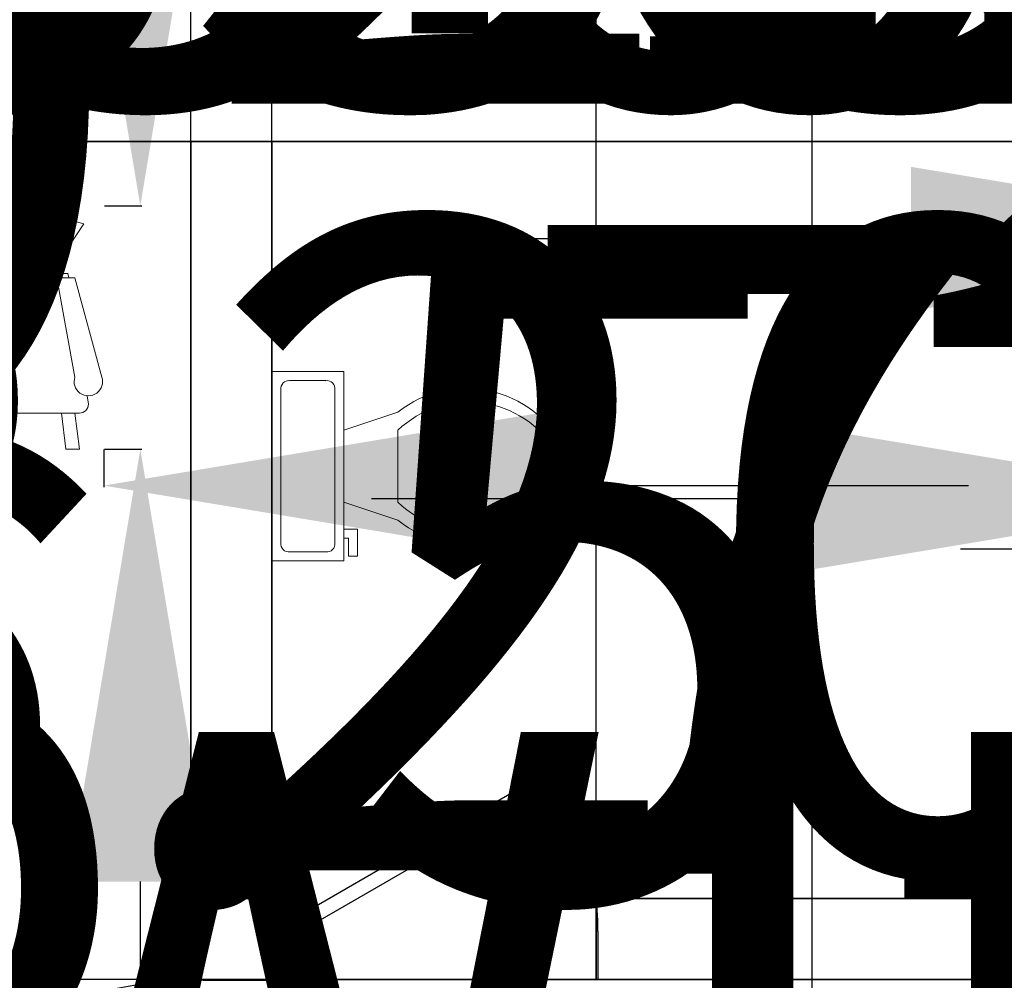
# Model space of a CAD drawing. Units: inches. Extents: x -307 to 2141, y -58 to 895.
# Tile 20 of 28: x 666 to 776, y 589 to 696. Entities that reach past the tile are written whole.
import ezdxf

# ---------------------------------------------------------------- set-up
doc = ezdxf.new("R2010")
doc.units = ezdxf.units.IN
doc.header["$MEASUREMENT"] = 0
for name, color, linetype, lineweight in [('A-ANNO-DIMS', 2, 'Continuous', 18), ('A-DOOR', 3, 'Continuous', 25), ('A-FLOR-FIXT', 9, 'Continuous', 18), ('A-FURN', 8, 'Continuous', 18), ('A-WALL', 7, 'Continuous', 35)]:
    doc.layers.add(name, color=color, linetype=linetype, lineweight=lineweight)
doc.styles.get("Standard").update_dxf_attribs({"font": 'arial.ttf'})
doc.dimstyles.get("Standard").update_dxf_attribs({"dimtxt": 72, "dimasz": 48, "dimexe": 0.18, "dimexo": 0.0625, "dimgap": 0.09, "dimtad": 0, "dimtih": 1, "dimtoh": 1, "dimdec": 0, "dimrnd": 48, "dimzin": 0, "dimdsep": 46, "dimlunit": 3, "dimtxsty": 'Standard', "dimcen": 0.09, "dimadec": 0, "dimazin": 0, "dimtfac": 1, "dimtdec": 0, "dimtofl": 0, "dimtmove": 0, "dimatfit": 3, "dimfxl": 1, "dimtolj": 1, "dimtzin": 0, "dimarcsym": 0})

# ---------------------------------------------------------------- blocks, each defined once
blk = doc.blocks.new('*U3')
for p, q in [((-40, 0), (-40, 6)), ((0, 0), (0, 6))]:
    blk.add_line(p, q)
blk.add_lwpolyline([(0, 0), (-34.641, -20), (-35.516, -18.484), (-0.875, 1.516)], close=True)
blk.add_arc((0, 0), 40, 180, 210)
blk = doc.blocks.new('*U4')
for p, q in [((-40, 0), (-40, 6)), ((0, 0), (0, 6))]:
    blk.add_line(p, q)
blk.add_lwpolyline([(0, 0), (-34.64, -20), (-35.52, -18.48), (-0.88, 1.52)], close=True)
blk.add_arc((0, 0), 40, 180, 210)
blk = doc.blocks.new('Toilet - top')
for p, q in [((9.5, -6), (9.5, -2)), ((-10, -8.5), (-8, -8.5)), ((-10, -9.5), (-10, -8.5)), ((-8, -8.5), (-8, -8)), ((-7, -8), (-7, -9.5)), ((-4, -8), (-6, -14)), ((4, -8), (6, -14)), ((-7, -9.5), (-10, -9.5)), ((4, -14), (-4, -14))]:
    blk.add_line(p, q)
blk.add_lwpolyline([(10.5, -8), (10.5, 0), (-10.5, 0), (-10.5, -8)], close=True)
for points in [[(8.5, -1), (-8.5, -1)], [(-9.5, -2), (-9.5, -6)], [(-8.5, -7), (8.5, -7)]]:
    blk.add_lwpolyline(points)
for centre, radius, start, end in [((-8.62, -1.88), 0.884, 81.8699, 188.1301), ((8.62, -1.88), 0.884, 351.8699, 98.1301), ((-8.62, -6.12), 0.884, 171.8699, 278.1301), ((8.62, -6.12), 0.884, 261.8699, 8.1301), ((3.52, -21.58), 12.17, 141.4691, 247.9714), ((4.2, -21.82), 11.33, 136.3677, 238.9468), ((-3.52, -21.58), 12.17, 292.0284, 38.5307), ((-4.2, -21.82), 11.33, 301.053, 43.6321), ((0, -27.88), 4, 245.7318, 294.2682), ((0, -29), 4, 254.8605, 285.1395)]:
    blk.add_arc(centre, radius, start, end)
blk = doc.blocks.new('Chair - Rocking')
for p, q in [((-8, -4.5), (-10, -1.5)), ((8, -4.5), (10, -1.5)), ((-4.5, -7), (-4.96674, -4.19951)), ((-4, -7), (-4.40532, -4.16272)), ((-1.5, -4.05012), (-1.5, -7)), ((-1, -7), (-1, -4.05012)), ((1, -7), (1, -4.04655)), ((1.5, -4.05012), (1.5, -7)), ((4, -7), (4.40187, -4.18694)), ((4.5, -7), (4.96761, -4.19437)), ((-7.5, -4.5), (-7, -7)), ((-6.5, -7), (-7.02225, -4.43)), ((6.5, -7), (7, -4.4057)), ((7.5, -4.5), (7, -7)), ((-9, -7.5), (-12, -18.49999)), ((-7, -7.5), (-9, -7.5)), ((-9, -18.49999), (-7, -7.5)), ((-8.23428, -6.99939), (-8.3093, -7.47958)), ((-8.23041, -7), (8.23915, -7)), ((7, -7.5), (9, -7.5)), ((9, -18.49999), (7, -7.5)), ((8.31071, -7.48854), (8.23449, -7.00073)), ((9, -7.5), (12, -18.49999)), ((-10.36644, -20.64523), (-10.5, -21.49999)), ((10.5, -21.49999), (10.3575, -20.58798)), ((-9, -22.49999), (-9.5, -26.49999)), ((0, -22.49999), (-9.5, -22.49999)), ((-8, -26.49999), (-7.5, -22.49999)), ((0, -22.49999), (9.5, -22.49999)), ((8, -26.49999), (7.5, -22.49999)), ((9, -22.49999), (9.5, -26.49999)), ((-9.5, -26.49999), (-8, -26.49999)), ((9.5, -26.49999), (8, -26.49999))]:
    blk.add_line(p, q)
for centre, radius, start, end in [((0, -34.08333), 34.08333, 72.93847, 107.0615), ((0, -68.25004), 64.25, 93.92211, 97.15267), ((0, -68.25004), 64.25, 82.84733, 93.92211), ((-10.5, -18.99999), 1.58114, 161.5651, 18.43495), ((10.5, -18.99999), 1.58114, 161.5651, 18.43495), ((-9.5, -21.49999), 1, 180, 270), ((9.5, -21.49999), 1, 270, 0)]:
    blk.add_arc(centre, radius, start, end)
blk = doc.blocks.new('*D26')
at = {"layer": 'A-ANNO-DIMS', "color": 0, "lineweight": -2, "transparency": 16777216}
for p, q in [((565.34, 584.2), (565.34, 572.08)), ((645.34, 584.2), (645.34, 572.08)), ((517.34, 572.26), (469.34, 572.26)), ((693.34, 572.26), (741.34, 572.26))]:
    blk.add_line(p, q, dxfattribs=at)
at = {"layer": 'A-ANNO-DIMS', "color": 0, "transparency": 16777216}
for points in [[(517.34, 580.26), (517.34, 564.26), (565.34, 572.26)], [(693.34, 580.26), (693.34, 564.26), (645.34, 572.26)]]:
    blk.add_solid(points, dxfattribs=at)
at = {"layer": 'Defpoints', "color": 0, "transparency": 16777216}
for p in [(565.34, 584.26), (645.34, 584.26), (565.34, 572.26)]:
    blk.add_point(p, dxfattribs=at)
at = {"layer": 'A-ANNO-DIMS', "color": 0, "transparency": 16777216, "insert": (178.23, 572.26), "char_height": 72, "attachment_point": 5}
blk.add_mtext('\\A1;BED 80 TYP.', dxfattribs=at)
blk = doc.blocks.new('*D30')
at = {"layer": 'A-ANNO-DIMS', "color": 0, "lineweight": -2, "transparency": 16777216}
for p, q in [((570.74, 532.83), (570.74, 580.83)), ((570.74, 580.83), (618.74, 580.83)), ((565.4, 484.83), (570.92, 484.83)), ((565.4, 448.83), (570.92, 448.83)), ((570.74, 400.83), (570.74, 352.83))]:
    blk.add_line(p, q, dxfattribs=at)
at = {"layer": 'A-ANNO-DIMS', "color": 0, "transparency": 16777216}
for points in [[(562.74, 532.83), (578.74, 532.83), (570.74, 484.83)], [(562.74, 400.83), (578.74, 400.83), (570.74, 448.83)]]:
    blk.add_solid(points, dxfattribs=at)
at = {"layer": 'Defpoints', "color": 0, "transparency": 16777216}
for p in [(565.34, 484.83), (570.74, 484.83), (565.34, 448.83)]:
    blk.add_point(p, dxfattribs=at)
at = {"layer": 'A-ANNO-DIMS', "color": 0, "transparency": 16777216, "insert": (1030.17, 580.83), "char_height": 72, "attachment_point": 5}
blk.add_mtext('\\A1;WINDOW 36 TYP.', dxfattribs=at)
blk = doc.blocks.new('*D32')
at = {"layer": 'A-ANNO-DIMS', "color": 0, "lineweight": -2, "transparency": 16777216}
for p, q in [((813.29, 682.28), (813.29, 671.36)), ((885.29, 682.28), (885.29, 671.36)), ((765.29, 671.54), (717.29, 671.54)), ((933.29, 671.54), (981.29, 671.54))]:
    blk.add_line(p, q, dxfattribs=at)
at = {"layer": 'A-ANNO-DIMS', "color": 0, "transparency": 16777216}
for points in [[(765.29, 679.54), (765.29, 663.54), (813.29, 671.54)], [(933.29, 679.54), (933.29, 663.54), (885.29, 671.54)]]:
    blk.add_solid(points, dxfattribs=at)
at = {"layer": 'Defpoints', "color": 0, "transparency": 16777216}
for p in [(813.29, 682.34), (885.29, 682.34), (885.29, 671.54)]:
    blk.add_point(p, dxfattribs=at)
at = {"layer": 'A-ANNO-DIMS', "color": 0, "transparency": 16777216, "insert": (1392.73, 671.54), "char_height": 72, "attachment_point": 5}
blk.add_mtext('\\A1;WINDOW 72 TYP.', dxfattribs=at)
blk = doc.blocks.new('*D36')
at = {"layer": 'A-ANNO-DIMS', "color": 0, "lineweight": -2, "transparency": 16777216}
for p, q in [((871.71, 562.4), (871.76, 610.4)), ((876.55, 514.4), (871.47, 514.4)), ((876.51, 481.35), (871.44, 481.36)), ((871.56, 433.36), (871.51, 385.36)), ((871.51, 385.36), (823.51, 385.36))]:
    blk.add_line(p, q, dxfattribs=at)
at = {"layer": 'A-ANNO-DIMS', "color": 0, "transparency": 16777216}
for points in [[(863.71, 562.41), (879.71, 562.4), (871.65, 514.4)], [(863.56, 433.37), (879.56, 433.35), (871.62, 481.36)]]:
    blk.add_solid(points, dxfattribs=at)
at = {"layer": 'Defpoints', "color": 0, "transparency": 16777216}
for p in [(876.61, 514.4), (871.62, 481.36), (876.57, 481.35)]:
    blk.add_point(p, dxfattribs=at)
at = {"layer": 'A-ANNO-DIMS', "color": 0, "transparency": 16777216, "insert": (548.95, 385.36), "char_height": 72, "attachment_point": 5}
blk.add_mtext('\\A1;WC 33 TYP.', dxfattribs=at)
blk = doc.blocks.new('*D37')
at = {"layer": 'A-ANNO-DIMS', "color": 0, "lineweight": -2, "transparency": 16777216}
for p, q in [((828.62, 519.41), (780.62, 519.46)), ((876.61, 514.46), (876.62, 519.54)), ((897.61, 514.44), (897.62, 519.51)), ((945.62, 519.28), (993.62, 519.22))]:
    blk.add_line(p, q, dxfattribs=at)
at = {"layer": 'A-ANNO-DIMS', "color": 0, "transparency": 16777216}
for points in [[(828.63, 527.41), (828.61, 511.41), (876.62, 519.36)], [(945.63, 527.28), (945.61, 511.28), (897.62, 519.33)]]:
    blk.add_solid(points, dxfattribs=at)
at = {"layer": 'Defpoints', "color": 0, "transparency": 16777216}
for p in [(876.62, 519.36), (876.61, 514.4), (897.61, 514.38)]:
    blk.add_point(p, dxfattribs=at)
at = {"layer": 'A-ANNO-DIMS', "color": 0, "transparency": 16777216, "insert": (604.68, 519.46), "char_height": 72, "attachment_point": 5}
blk.add_mtext('\\A1;21 TYP.', dxfattribs=at)
blk = doc.blocks.new('*D42')
at = {"layer": 'A-ANNO-DIMS', "color": 0, "lineweight": -2, "transparency": 16777216}
for p, q in [((880.26, 543.86), (928.25, 544.87)), ((822.3, 541.2), (822.27, 542.82)), ((832.3, 541.41), (832.27, 543.03)), ((774.28, 541.63), (726.29, 540.62))]:
    blk.add_line(p, q, dxfattribs=at)
at = {"layer": 'A-ANNO-DIMS', "color": 0, "transparency": 16777216}
for points in [[(880.09, 551.86), (880.43, 535.86), (832.27, 542.85)], [(774.11, 549.63), (774.45, 533.63), (822.27, 542.64)]]:
    blk.add_solid(points, dxfattribs=at)
at = {"layer": 'Defpoints', "color": 0, "transparency": 16777216}
for p in [(832.27, 542.85), (832.3, 541.35), (822.3, 541.14)]:
    blk.add_point(p, dxfattribs=at)
at = {"layer": 'A-ANNO-DIMS', "color": 0, "transparency": 16777216, "insert": (1192.89, 544.87), "char_height": 72, "attachment_point": 5}
blk.add_mtext('\\A1;FAUCET 10', dxfattribs=at)
blk = doc.blocks.new('*D43')
at = {"layer": 'A-ANNO-DIMS', "color": 0, "lineweight": -2, "transparency": 16777216}
for p, q in [((818.79, 637.09), (770.79, 637.09)), ((819.79, 589.1), (818.79, 637.09)), ((822.24, 541.14), (820.62, 541.1)), ((822.38, 534.64), (820.76, 534.61)), ((821.95, 486.62), (822.96, 438.63))]:
    blk.add_line(p, q, dxfattribs=at)
at = {"layer": 'A-ANNO-DIMS', "color": 0, "transparency": 16777216}
for points in [[(827.79, 589.27), (811.8, 588.93), (820.8, 541.11)], [(829.95, 486.79), (813.95, 486.45), (820.94, 534.61)]]:
    blk.add_solid(points, dxfattribs=at)
at = {"layer": 'Defpoints', "color": 0, "transparency": 16777216}
for p in [(820.8, 541.11), (822.3, 541.14), (822.44, 534.64)]:
    blk.add_point(p, dxfattribs=at)
at = {"layer": 'A-ANNO-DIMS', "color": 0, "transparency": 16777216, "insert": (747.39, 637.09), "char_height": 72, "attachment_point": 5}
blk.add_mtext('\\A1;7', dxfattribs=at)
blk = doc.blocks.new('*D44')
at = {"layer": 'A-ANNO-DIMS', "color": 0, "lineweight": -2, "transparency": 16777216}
for p, q in [((815.33, 520.71), (815.41, 516.91)), ((839.87, 521.22), (839.95, 517.42)), ((887.94, 518.61), (935.93, 519.62)), ((767.41, 516.08), (719.42, 515.07))]:
    blk.add_line(p, q, dxfattribs=at)
at = {"layer": 'A-ANNO-DIMS', "color": 0, "transparency": 16777216}
for points in [[(887.77, 526.61), (888.11, 510.61), (839.95, 517.6)], [(767.25, 524.08), (767.58, 508.08), (815.4, 517.09)]]:
    blk.add_solid(points, dxfattribs=at)
at = {"layer": 'Defpoints', "color": 0, "transparency": 16777216}
for p in [(815.33, 520.77), (839.87, 521.29), (839.95, 517.6)]:
    blk.add_point(p, dxfattribs=at)
at = {"layer": 'A-ANNO-DIMS', "color": 0, "transparency": 16777216, "insert": (1151.16, 519.62), "char_height": 72, "attachment_point": 5}
blk.add_mtext('\\A1;BASIN 25', dxfattribs=at)
blk = doc.blocks.new('*D45')
at = {"layer": 'A-ANNO-DIMS', "color": 0, "lineweight": -2, "transparency": 16777216}
for p, q in [((841.11, 637.47), (793.11, 637.47)), ((842.12, 589.48), (841.11, 637.47)), ((839.51, 541.42), (843.31, 541.5)), ((839.93, 521.29), (843.73, 521.37)), ((844.56, 473.37), (845.57, 425.38))]:
    blk.add_line(p, q, dxfattribs=at)
at = {"layer": 'A-ANNO-DIMS', "color": 0, "transparency": 16777216}
for points in [[(850.12, 589.65), (834.12, 589.32), (843.13, 541.49)], [(852.56, 473.54), (836.56, 473.21), (843.55, 521.36)]]:
    blk.add_solid(points, dxfattribs=at)
at = {"layer": 'Defpoints', "color": 0, "transparency": 16777216}
for p in [(839.45, 541.42), (843.13, 541.49), (839.87, 521.29)]:
    blk.add_point(p, dxfattribs=at)
at = {"layer": 'A-ANNO-DIMS', "color": 0, "transparency": 16777216, "insert": (740.96, 637.47), "char_height": 72, "attachment_point": 5}
blk.add_mtext('\\A1;20', dxfattribs=at)
blk = doc.blocks.new('*D46')
at = {"layer": 'A-ANNO-DIMS', "color": 0, "lineweight": -2, "transparency": 16777216}
for p, q in [((801.41, 645.78), (801.41, 642.52)), ((822.41, 645.78), (822.41, 642.52)), ((753.41, 642.7), (705.41, 642.7)), ((870.41, 642.7), (918.41, 642.7))]:
    blk.add_line(p, q, dxfattribs=at)
at = {"layer": 'A-ANNO-DIMS', "color": 0, "transparency": 16777216}
for points in [[(753.41, 650.7), (753.41, 634.7), (801.41, 642.7)], [(870.41, 650.7), (870.41, 634.7), (822.41, 642.7)]]:
    blk.add_solid(points, dxfattribs=at)
at = {"layer": 'Defpoints', "color": 0, "transparency": 16777216}
for p in [(801.41, 645.85), (822.41, 645.85), (822.41, 642.7)]:
    blk.add_point(p, dxfattribs=at)
at = {"layer": 'A-ANNO-DIMS', "color": 0, "transparency": 16777216, "insert": (1282.7, 642.7), "char_height": 72, "attachment_point": 5}
blk.add_mtext('\\A1;DESK CHAIR 21', dxfattribs=at)
blk = doc.blocks.new('*D52')
at = {"layer": 'A-ANNO-DIMS', "color": 0, "lineweight": -2, "transparency": 16777216}
for p, q in [((660.21, 554.25), (660.21, 602.25)), ((673.8, 506.25), (660.03, 506.25)), ((673.8, 415.25), (660.03, 415.25)), ((660.21, 367.25), (660.21, 319.25))]:
    blk.add_line(p, q, dxfattribs=at)
at = {"layer": 'A-ANNO-DIMS', "color": 0, "transparency": 16777216}
for points in [[(652.21, 554.25), (668.21, 554.25), (660.21, 506.25)], [(652.21, 367.25), (668.21, 367.25), (660.21, 415.25)]]:
    blk.add_solid(points, dxfattribs=at)
at = {"layer": 'Defpoints', "color": 0, "transparency": 16777216}
for p in [(673.86, 506.25), (660.21, 415.25), (673.86, 415.25)]:
    blk.add_point(p, dxfattribs=at)
at = {"layer": 'A-ANNO-DIMS', "color": 0, "transparency": 16777216, "insert": (660.21, 460.75), "char_height": 72, "attachment_point": 5}
blk.add_mtext('\\A1;DINING SET 91', dxfattribs=at)
blk = doc.blocks.new('*D56')
at = {"layer": 'A-ANNO-DIMS', "color": 0, "lineweight": -2, "transparency": 16777216}
for p, q in [((679.73, 723.21), (679.73, 771.21)), ((679.73, 771.21), (727.73, 771.21)), ((675.74, 675.21), (679.91, 675.21)), ((675.74, 648.21), (679.91, 648.21)), ((679.73, 600.21), (679.73, 552.21))]:
    blk.add_line(p, q, dxfattribs=at)
at = {"layer": 'A-ANNO-DIMS', "color": 0, "transparency": 16777216}
for points in [[(671.73, 723.21), (687.73, 723.21), (679.73, 675.21)], [(671.73, 600.21), (687.73, 600.21), (679.73, 648.21)]]:
    blk.add_solid(points, dxfattribs=at)
at = {"layer": 'Defpoints', "color": 0, "transparency": 16777216}
for p in [(675.68, 675.21), (679.73, 675.21), (675.68, 648.21)]:
    blk.add_point(p, dxfattribs=at)
at = {"layer": 'A-ANNO-DIMS', "color": 0, "transparency": 16777216, "insert": (1006.66, 771.21), "char_height": 72, "attachment_point": 5}
blk.add_mtext('\\A1;ROCKER 27', dxfattribs=at)
blk = doc.blocks.new('*D57')
at = {"layer": 'A-ANNO-DIMS', "color": 0, "lineweight": -2, "transparency": 16777216}
for p, q in [((651.25, 648.15), (651.25, 643.98)), ((675.68, 648.15), (675.68, 643.98)), ((603.25, 644.16), (555.25, 644.16)), ((723.68, 644.16), (771.68, 644.16))]:
    blk.add_line(p, q, dxfattribs=at)
at = {"layer": 'A-ANNO-DIMS', "color": 0, "transparency": 16777216}
for points in [[(603.25, 652.16), (603.25, 636.16), (651.25, 644.16)], [(723.68, 652.16), (723.68, 636.16), (675.68, 644.16)]]:
    blk.add_solid(points, dxfattribs=at)
at = {"layer": 'Defpoints', "color": 0, "transparency": 16777216}
for p in [(651.25, 648.21), (675.68, 648.21), (675.68, 644.16)]:
    blk.add_point(p, dxfattribs=at)
at = {"layer": 'A-ANNO-DIMS', "color": 0, "transparency": 16777216, "insert": (823.81, 644.16), "char_height": 72, "attachment_point": 5}
blk.add_mtext('\\A1;24', dxfattribs=at)
blk = doc.blocks.new('*D62')
at = {"layer": 'A-ANNO-DIMS', "color": 0, "lineweight": -2, "transparency": 16777216}
for p, q in [((556.34, 691.4), (556.34, 722.72)), ((916.34, 490.97), (916.34, 722.72)), ((604.34, 722.54), (656.85, 722.54)), ((868.34, 722.54), (815.82, 722.54))]:
    blk.add_line(p, q, dxfattribs=at)
at = {"layer": 'A-ANNO-DIMS', "color": 0, "transparency": 16777216}
for points in [[(604.34, 730.54), (604.34, 714.54), (556.34, 722.54)], [(868.34, 730.54), (868.34, 714.54), (916.34, 722.54)]]:
    blk.add_solid(points, dxfattribs=at)
at = {"layer": 'Defpoints', "color": 0, "transparency": 16777216}
for p in [(916.34, 722.54), (556.34, 691.34), (916.34, 490.9)]:
    blk.add_point(p, dxfattribs=at)
at = {"layer": 'A-ANNO-DIMS', "color": 0, "transparency": 16777216, "insert": (736.34, 722.54), "char_height": 72, "attachment_point": 5}
blk.add_mtext('\\A1;360', dxfattribs=at)
blk = doc.blocks.new('*D63')
at = {"layer": 'A-ANNO-DIMS', "color": 0, "lineweight": -2, "transparency": 16777216}
for p, q in [((916.4, 691.34), (947.72, 691.34)), ((947.54, 643.34), (947.54, 416.19)), ((947.54, 115.34), (947.54, 342.49)), ((704.68, 67.34), (947.72, 67.34))]:
    blk.add_line(p, q, dxfattribs=at)
at = {"layer": 'A-ANNO-DIMS', "color": 0, "transparency": 16777216}
for points in [[(939.54, 643.34), (955.54, 643.34), (947.54, 691.34)], [(939.54, 115.34), (955.54, 115.34), (947.54, 67.34)]]:
    blk.add_solid(points, dxfattribs=at)
at = {"layer": 'Defpoints', "color": 0, "transparency": 16777216}
for p in [(916.34, 691.34), (704.62, 67.34), (947.54, 67.34)]:
    blk.add_point(p, dxfattribs=at)
at = {"layer": 'A-ANNO-DIMS', "color": 0, "transparency": 16777216, "insert": (947.54, 379.34), "char_height": 72, "attachment_point": 5}
blk.add_mtext('\\A1;624', dxfattribs=at)
blk = doc.blocks.new('*D68')
at = {"layer": 'A-ANNO-DIMS', "color": 0, "lineweight": -2, "transparency": 16777216}
for p, q in [((525.13, 586.34), (525.13, 634.34)), ((525.13, 634.34), (573.13, 634.34)), ((565.27, 538.34), (524.95, 538.34)), ((556.27, 484.83), (524.95, 484.83)), ((525.13, 436.83), (525.13, 388.83))]:
    blk.add_line(p, q, dxfattribs=at)
at = {"layer": 'A-ANNO-DIMS', "color": 0, "transparency": 16777216}
for points in [[(517.13, 586.34), (533.13, 586.34), (525.13, 538.34)], [(517.13, 436.83), (533.13, 436.83), (525.13, 484.83)]]:
    blk.add_solid(points, dxfattribs=at)
at = {"layer": 'Defpoints', "color": 0, "transparency": 16777216}
for p in [(525.13, 538.34), (565.34, 538.34), (556.34, 484.83)]:
    blk.add_point(p, dxfattribs=at)
at = {"layer": 'A-ANNO-DIMS', "color": 0, "transparency": 16777216, "insert": (687.75, 634.34), "char_height": 72, "attachment_point": 5}
blk.add_mtext('\\A1;53.51', dxfattribs=at)
blk = doc.blocks.new('*D69')
at = {"layer": 'A-ANNO-DIMS', "color": 0, "lineweight": -2, "transparency": 16777216}
for p, q in [((525.13, 682.34), (525.13, 730.34)), ((525.13, 730.34), (573.13, 730.34)), ((565.27, 682.34), (524.95, 682.34)), ((525.13, 586.34), (525.13, 634.34)), ((565.27, 538.34), (524.95, 538.34))]:
    blk.add_line(p, q, dxfattribs=at)
at = {"layer": 'A-ANNO-DIMS', "color": 0, "transparency": 16777216}
for points in [[(517.13, 634.34), (533.13, 634.34), (525.13, 682.34)], [(517.13, 586.34), (533.13, 586.34), (525.13, 538.34)]]:
    blk.add_solid(points, dxfattribs=at)
at = {"layer": 'Defpoints', "color": 0, "transparency": 16777216}
for p in [(525.13, 682.34), (565.34, 682.34), (565.34, 538.34)]:
    blk.add_point(p, dxfattribs=at)
at = {"layer": 'A-ANNO-DIMS', "color": 0, "transparency": 16777216, "insert": (649.22, 730.34), "char_height": 72, "attachment_point": 5}
blk.add_mtext('\\A1;144', dxfattribs=at)
blk = doc.blocks.new('*D75')
at = {"layer": 'A-ANNO-DIMS', "color": 0, "lineweight": -2, "transparency": 16777216}
for p, q in [((565.34, 682.4), (565.34, 722.72)), ((685.34, 682.4), (685.34, 722.72)), ((613.34, 722.54), (637.34, 722.54)), ((685.34, 722.54), (733.34, 722.54))]:
    blk.add_line(p, q, dxfattribs=at)
at = {"layer": 'A-ANNO-DIMS', "color": 0, "transparency": 16777216}
for points in [[(613.34, 730.54), (613.34, 714.54), (565.34, 722.54)], [(637.34, 730.54), (637.34, 714.54), (685.34, 722.54)]]:
    blk.add_solid(points, dxfattribs=at)
at = {"layer": 'Defpoints', "color": 0, "transparency": 16777216}
for p in [(685.34, 722.54), (565.34, 682.34), (685.34, 682.34)]:
    blk.add_point(p, dxfattribs=at)
at = {"layer": 'A-ANNO-DIMS', "color": 0, "transparency": 16777216, "insert": (809.45, 722.54), "char_height": 72, "attachment_point": 5}
blk.add_mtext('\\A1;120', dxfattribs=at)
blk = doc.blocks.new('*D76')
at = {"layer": 'A-ANNO-DIMS', "color": 0, "lineweight": -2, "transparency": 16777216}
for p, q in [((694.34, 682.4), (694.34, 722.72)), ((778.34, 682.4), (778.34, 722.72)), ((646.34, 722.54), (598.34, 722.54)), ((826.34, 722.54), (874.34, 722.54))]:
    blk.add_line(p, q, dxfattribs=at)
at = {"layer": 'A-ANNO-DIMS', "color": 0, "transparency": 16777216}
for points in [[(646.34, 730.54), (646.34, 714.54), (694.34, 722.54)], [(826.34, 730.54), (826.34, 714.54), (778.34, 722.54)]]:
    blk.add_solid(points, dxfattribs=at)
at = {"layer": 'Defpoints', "color": 0, "transparency": 16777216}
for p in [(778.34, 722.54), (694.34, 682.34), (778.34, 682.34)]:
    blk.add_point(p, dxfattribs=at)
at = {"layer": 'A-ANNO-DIMS', "color": 0, "transparency": 16777216, "insert": (925.9, 722.54), "char_height": 72, "attachment_point": 5}
blk.add_mtext('\\A1;84', dxfattribs=at)
blk = doc.blocks.new('*D78')
at = {"layer": 'A-ANNO-DIMS', "color": 0, "lineweight": -2, "transparency": 16777216}
for p, q in [((947.53984, 730.340828), (947.53984, 778.340828)), ((778.39834, 682.340828), (947.71984, 682.340828)), ((730.39834, 598.340828), (947.71984, 598.340828)), ((947.53984, 550.340828), (947.53984, 502.340828))]:
    blk.add_line(p, q, dxfattribs=at)
at = {"layer": 'A-ANNO-DIMS', "color": 0, "transparency": 16777216}
for points in [[(939.53984, 730.340828), (955.53984, 730.340828), (947.53984, 682.340828)], [(939.53984, 550.340828), (955.53984, 550.340828), (947.53984, 598.340828)]]:
    blk.add_solid(points, dxfattribs=at)
at = {"layer": 'Defpoints', "color": 0, "transparency": 16777216}
for p in [(778.33584, 682.340828), (947.53984, 682.340828), (730.33584, 598.340828)]:
    blk.add_point(p, dxfattribs=at)
at = {"layer": 'A-ANNO-DIMS', "color": 0, "transparency": 16777216, "insert": (947.53984, 640.340828), "char_height": 72, "attachment_point": 5}
blk.add_mtext('\\A1;84', dxfattribs=at)
blk = doc.blocks.new('*D80')
at = {"layer": 'A-ANNO-DIMS', "color": 0, "lineweight": -2, "transparency": 16777216}
for p, q in [((811.34, 517.4), (811.34, 722.72)), ((907.34, 541.4), (907.34, 722.72)), ((763.34, 722.54), (715.34, 722.54)), ((955.34, 722.54), (1003.34, 722.54))]:
    blk.add_line(p, q, dxfattribs=at)
at = {"layer": 'A-ANNO-DIMS', "color": 0, "transparency": 16777216}
for points in [[(763.34, 730.54), (763.34, 714.54), (811.34, 722.54)], [(955.34, 730.54), (955.34, 714.54), (907.34, 722.54)]]:
    blk.add_solid(points, dxfattribs=at)
at = {"layer": 'Defpoints', "color": 0, "transparency": 16777216}
for p in [(907.34, 722.54), (907.34, 541.34), (811.34, 517.34)]:
    blk.add_point(p, dxfattribs=at)
at = {"layer": 'A-ANNO-DIMS', "color": 0, "transparency": 16777216, "insert": (1054.97, 722.54), "char_height": 72, "attachment_point": 5}
blk.add_mtext('\\A1;96', dxfattribs=at)
blk = doc.blocks.new('*D82')
at = {"layer": 'A-ANNO-DIMS', "color": 0, "lineweight": -2, "transparency": 16777216}
for p, q in [((525.13, 565.34), (525.13, 613.34)), ((525.13, 613.34), (573.13, 613.34)), ((802.27, 517.34), (524.95, 517.34)), ((802.27, 481.34), (524.95, 481.34)), ((525.13, 433.34), (525.13, 385.34))]:
    blk.add_line(p, q, dxfattribs=at)
at = {"layer": 'A-ANNO-DIMS', "color": 0, "transparency": 16777216}
for points in [[(517.13, 565.34), (533.13, 565.34), (525.13, 517.34)], [(517.13, 433.34), (533.13, 433.34), (525.13, 481.34)]]:
    blk.add_solid(points, dxfattribs=at)
at = {"layer": 'Defpoints', "color": 0, "transparency": 16777216}
for p in [(525.13, 517.34), (802.34, 517.34), (802.34, 481.34)]:
    blk.add_point(p, dxfattribs=at)
at = {"layer": 'A-ANNO-DIMS', "color": 0, "transparency": 16777216, "insert": (624.74, 613.34), "char_height": 72, "attachment_point": 5}
blk.add_mtext('\\A1;36', dxfattribs=at)
blk = doc.blocks.new('*D88')
at = {"layer": 'A-ANNO-DIMS', "color": 0, "lineweight": -2, "transparency": 16777216}
for p, q in [((565.33584, 295.403328), (565.33584, 722.724828)), ((754.33584, 271.403328), (754.33584, 722.724828)), ((517.33584, 722.544828), (469.33584, 722.544828)), ((802.33584, 722.544828), (850.33584, 722.544828))]:
    blk.add_line(p, q, dxfattribs=at)
at = {"layer": 'A-ANNO-DIMS', "color": 0, "transparency": 16777216}
for points in [[(517.33584, 730.544828), (517.33584, 714.544828), (565.33584, 722.544828)], [(802.33584, 730.544828), (802.33584, 714.544828), (754.33584, 722.544828)]]:
    blk.add_solid(points, dxfattribs=at)
at = {"layer": 'Defpoints', "color": 0, "transparency": 16777216}
for p in [(754.33584, 722.544828), (565.33584, 295.340828), (754.33584, 271.340828)]:
    blk.add_point(p, dxfattribs=at)
at = {"layer": 'A-ANNO-DIMS', "color": 0, "transparency": 16777216, "insert": (659.83584, 722.544828), "char_height": 72, "attachment_point": 5}
blk.add_mtext('\\A1;189', dxfattribs=at)
blk = doc.blocks.new('*D94')
at = {"layer": 'A-ANNO-DIMS', "color": 0, "lineweight": -2, "transparency": 16777216}
for p, q in [((565.34, 529.4), (565.34, 722.72)), ((629.84, 529.4), (629.84, 722.72)), ((517.34, 722.54), (469.34, 722.54)), ((677.84, 722.54), (725.84, 722.54))]:
    blk.add_line(p, q, dxfattribs=at)
at = {"layer": 'A-ANNO-DIMS', "color": 0, "transparency": 16777216}
for points in [[(517.34, 730.54), (517.34, 714.54), (565.34, 722.54)], [(677.84, 730.54), (677.84, 714.54), (629.84, 722.54)]]:
    blk.add_solid(points, dxfattribs=at)
at = {"layer": 'Defpoints', "color": 0, "transparency": 16777216}
for p in [(629.84, 722.54), (565.34, 529.34), (629.84, 529.34)]:
    blk.add_point(p, dxfattribs=at)
at = {"layer": 'A-ANNO-DIMS', "color": 0, "transparency": 16777216, "insert": (819.9, 722.54), "char_height": 72, "attachment_point": 5}
blk.add_mtext('\\A1;64.5', dxfattribs=at)
blk = doc.blocks.new('*D95')
at = {"layer": 'A-ANNO-DIMS', "color": 0, "lineweight": -2, "transparency": 16777216}
for p, q in [((947.54, 577.34), (947.54, 625.34)), ((947.54, 625.34), (995.54, 625.34)), ((629.9, 529.34), (947.72, 529.34)), ((629.9, 502.66), (947.72, 502.66)), ((947.54, 454.66), (947.54, 406.66))]:
    blk.add_line(p, q, dxfattribs=at)
at = {"layer": 'A-ANNO-DIMS', "color": 0, "transparency": 16777216}
for points in [[(939.54, 577.34), (955.54, 577.34), (947.54, 529.34)], [(939.54, 454.66), (955.54, 454.66), (947.54, 502.66)]]:
    blk.add_solid(points, dxfattribs=at)
at = {"layer": 'Defpoints', "color": 0, "transparency": 16777216}
for p in [(629.84, 529.34), (947.54, 529.34), (629.84, 502.66)]:
    blk.add_point(p, dxfattribs=at)
at = {"layer": 'A-ANNO-DIMS', "color": 0, "transparency": 16777216, "insert": (1117.8, 625.34), "char_height": 72, "attachment_point": 5}
blk.add_mtext('\\A1;26.68', dxfattribs=at)
blk = doc.blocks.new('*D96')
at = {"layer": 'A-ANNO-DIMS', "color": 0, "lineweight": -2, "transparency": 16777216}
for p, q in [((694.34, 598.4), (694.34, 722.72)), ((730.34, 598.4), (730.34, 722.72)), ((646.34, 722.54), (598.34, 722.54)), ((778.34, 722.54), (826.34, 722.54))]:
    blk.add_line(p, q, dxfattribs=at)
at = {"layer": 'A-ANNO-DIMS', "color": 0, "transparency": 16777216}
for points in [[(646.34, 730.54), (646.34, 714.54), (694.34, 722.54)], [(778.34, 730.54), (778.34, 714.54), (730.34, 722.54)]]:
    blk.add_solid(points, dxfattribs=at)
at = {"layer": 'Defpoints', "color": 0, "transparency": 16777216}
for p in [(730.34, 722.54), (694.34, 598.34), (730.34, 598.34)]:
    blk.add_point(p, dxfattribs=at)
at = {"layer": 'A-ANNO-DIMS', "color": 0, "transparency": 16777216, "insert": (877.95, 722.54), "char_height": 72, "attachment_point": 5}
blk.add_mtext('\\A1;36', dxfattribs=at)
blk = doc.blocks.new('*D97')
at = {"layer": 'A-ANNO-DIMS', "color": 0, "lineweight": -2, "transparency": 16777216}
for p, q in [((947.54, 637.34), (947.54, 685.34)), ((947.54, 685.34), (995.54, 685.34)), ((685.4, 589.34), (947.72, 589.34)), ((685.4, 538.34), (947.72, 538.34)), ((947.54, 490.34), (947.54, 442.34))]:
    blk.add_line(p, q, dxfattribs=at)
at = {"layer": 'A-ANNO-DIMS', "color": 0, "transparency": 16777216}
for points in [[(939.54, 637.34), (955.54, 637.34), (947.54, 589.34)], [(939.54, 490.34), (955.54, 490.34), (947.54, 538.34)]]:
    blk.add_solid(points, dxfattribs=at)
at = {"layer": 'Defpoints', "color": 0, "transparency": 16777216}
for p in [(685.34, 589.34), (947.54, 589.34), (685.34, 538.34)]:
    blk.add_point(p, dxfattribs=at)
at = {"layer": 'A-ANNO-DIMS', "color": 0, "transparency": 16777216, "insert": (1040.25, 685.34), "char_height": 72, "attachment_point": 5}
blk.add_mtext('\\A1;51', dxfattribs=at)
blk = doc.blocks.new('*D98')
at = {"layer": 'A-ANNO-DIMS', "color": 0, "lineweight": -2, "transparency": 16777216}
for p, q in [((525.13, 637.34), (525.13, 685.34)), ((525.13, 685.34), (573.13, 685.34)), ((787.27, 589.34), (524.95, 589.34)), ((787.27, 550.34), (524.95, 550.34)), ((525.13, 502.34), (525.13, 454.34))]:
    blk.add_line(p, q, dxfattribs=at)
at = {"layer": 'A-ANNO-DIMS', "color": 0, "transparency": 16777216}
for points in [[(517.13, 637.34), (533.13, 637.34), (525.13, 589.34)], [(517.13, 502.34), (533.13, 502.34), (525.13, 550.34)]]:
    blk.add_solid(points, dxfattribs=at)
at = {"layer": 'Defpoints', "color": 0, "transparency": 16777216}
for p in [(525.13, 589.34), (787.34, 589.34), (787.34, 550.34)]:
    blk.add_point(p, dxfattribs=at)
at = {"layer": 'A-ANNO-DIMS', "color": 0, "transparency": 16777216, "insert": (624.84, 685.34), "char_height": 72, "attachment_point": 5}
blk.add_mtext('\\A1;39', dxfattribs=at)
blk = doc.blocks.new('*D101')
at = {"layer": 'A-ANNO-DIMS', "color": 0, "lineweight": -2, "transparency": 16777216}
for p, q in [((556.34, 691.4), (556.34, 722.72)), ((589.36, 691.4), (589.36, 722.72)), ((508.34, 722.54), (460.34, 722.54)), ((637.36, 722.54), (685.36, 722.54))]:
    blk.add_line(p, q, dxfattribs=at)
at = {"layer": 'A-ANNO-DIMS', "color": 0, "transparency": 16777216}
for points in [[(508.34, 730.54), (508.34, 714.54), (556.34, 722.54)], [(637.36, 730.54), (637.36, 714.54), (589.36, 722.54)]]:
    blk.add_solid(points, dxfattribs=at)
at = {"layer": 'Defpoints', "color": 0, "transparency": 16777216}
for p in [(589.36, 722.54), (556.34, 691.34), (589.36, 691.34)]:
    blk.add_point(p, dxfattribs=at)
at = {"layer": 'A-ANNO-DIMS', "color": 0, "transparency": 16777216, "insert": (806.54, 722.54), "char_height": 72, "attachment_point": 5}
blk.add_mtext('\\A1;33.02', dxfattribs=at)
blk = doc.blocks.new('*D103')
at = {"layer": 'A-ANNO-DIMS', "color": 0, "lineweight": -2, "transparency": 16777216}
for p, q in [((685.34, 682.4), (685.34, 722.72)), ((694.34, 682.4), (694.34, 722.72)), ((637.34, 722.54), (589.34, 722.54)), ((742.34, 722.54), (790.34, 722.54))]:
    blk.add_line(p, q, dxfattribs=at)
at = {"layer": 'A-ANNO-DIMS', "color": 0, "transparency": 16777216}
for points in [[(637.34, 730.54), (637.34, 714.54), (685.34, 722.54)], [(742.34, 730.54), (742.34, 714.54), (694.34, 722.54)]]:
    blk.add_solid(points, dxfattribs=at)
at = {"layer": 'Defpoints', "color": 0, "transparency": 16777216}
for p in [(694.34, 722.54), (685.34, 682.34), (694.34, 682.34)]:
    blk.add_point(p, dxfattribs=at)
at = {"layer": 'A-ANNO-DIMS', "color": 0, "transparency": 16777216, "insert": (814.1, 722.54), "char_height": 72, "attachment_point": 5}
blk.add_mtext('\\A1;9', dxfattribs=at)
blk = doc.blocks.new('*D107')
at = {"layer": 'A-ANNO-DIMS', "color": 0, "lineweight": -2, "transparency": 16777216}
for p, q in [((565.34, 409.4), (565.34, 722.72)), ((589.34, 409.4), (589.34, 722.72)), ((517.34, 722.54), (469.34, 722.54)), ((637.34, 722.54), (685.34, 722.54))]:
    blk.add_line(p, q, dxfattribs=at)
at = {"layer": 'A-ANNO-DIMS', "color": 0, "transparency": 16777216}
for points in [[(517.34, 730.54), (517.34, 714.54), (565.34, 722.54)], [(637.34, 730.54), (637.34, 714.54), (589.34, 722.54)]]:
    blk.add_solid(points, dxfattribs=at)
at = {"layer": 'Defpoints', "color": 0, "transparency": 16777216}
for p in [(589.34, 722.54), (565.34, 409.34), (589.34, 409.34)]:
    blk.add_point(p, dxfattribs=at)
at = {"layer": 'A-ANNO-DIMS', "color": 0, "transparency": 16777216, "insert": (835.49, 722.54), "char_height": 72, "attachment_point": 5}
blk.add_mtext('\\A1;24.003', dxfattribs=at)
blk = doc.blocks.new('*D108')
at = {"layer": 'A-ANNO-DIMS', "color": 0, "lineweight": -2, "transparency": 16777216}
for p, q in [((947.54, 550.66), (947.54, 598.66)), ((589.4, 502.66), (947.72, 502.66)), ((589.4, 409.34), (947.72, 409.34)), ((947.54, 361.34), (947.54, 313.34))]:
    blk.add_line(p, q, dxfattribs=at)
at = {"layer": 'A-ANNO-DIMS', "color": 0, "transparency": 16777216}
for points in [[(939.54, 550.66), (955.54, 550.66), (947.54, 502.66)], [(939.54, 361.34), (955.54, 361.34), (947.54, 409.34)]]:
    blk.add_solid(points, dxfattribs=at)
at = {"layer": 'Defpoints', "color": 0, "transparency": 16777216}
for p in [(589.34, 502.66), (947.54, 502.66), (589.34, 409.34)]:
    blk.add_point(p, dxfattribs=at)
at = {"layer": 'A-ANNO-DIMS', "color": 0, "transparency": 16777216, "insert": (947.54, 456), "char_height": 72, "attachment_point": 5}
blk.add_mtext('\\A1;93.32', dxfattribs=at)

msp = doc.modelspace()

# ---------------------------------------------------------------- linework, layer by layer
at = {"layer": 'A-WALL'}
for p, q in [((916.3358, 691.3408), (556.3358, 691.3408)), ((907.3358, 682.3408), (565.3358, 682.3408)), ((685.3358, 682.3408), (685.3358, 589.3408)), ((694.3358, 682.3408), (694.3358, 589.3408)), ((694.3358, 598.3408), (685.3358, 598.3408)), ((787.3358, 598.3408), (730.3358, 598.3408)), ((730.3358, 598.3408), (730.3358, 589.3408)), ((694.3358, 589.3408), (685.3358, 589.3408)), ((787.3358, 589.3408), (730.3358, 589.3408))]:
    msp.add_line(p, q, dxfattribs=at)

# ---------------------------------------------------------------- block references
at = {"layer": 'A-DOOR'}
for name, p, xscale, yscale, zscale, rotation in [('*U4', (694.3358, 594.684), 0.9050111624103315, 0.9050111624103315, 0.9050111624103315, 180), ('*U3', (686.6989, 538.3408), 1.272826874134829, 1.272826874134829, 1.272826874134829, 270)]:
    msp.add_blockref(name, p, dxfattribs=dict(at, xscale=xscale, yscale=yscale, zscale=zscale, rotation=rotation))
at = {"layer": 'A-FLOR-FIXT', "rotation": 90}
msp.add_blockref('Toilet - top', (694.3358, 646.3094), dxfattribs=at)
at = {"layer": 'A-FURN'}
msp.add_blockref('Chair - Rocking', (663.4642, 674.711), dxfattribs=at)

# ---------------------------------------------------------------- dimensions: what is measured, and where the dimension line sits
at = {"layer": 'A-ANNO-DIMS'}
for base, p1, p2, angle, text, picture, middle in [((679.7317, 675.211), (675.6817, 648.211), (675.6817, 675.211), 90, 'ROCKER <>', '*D56', (1006.6621, 771.211)), ((570.7358, 484.8333), (565.3358, 448.8333), (565.3358, 484.8333), 90, 'WINDOW <> TYP.', '*D30', (1030.1737, 580.8333)), ((565.3358, 572.2648), (645.3359, 584.2648), (565.3358, 584.2648), 180, 'BED <> TYP.', '*D26', (178.2254, 572.2648)), ((832.2692, 542.8502), (822.3029, 541.1403), (832.3007, 541.3505), 1.204628, 'FAUCET <>', '*D42', (1192.8864, 544.8684)), ((660.2083, 415.2485), (673.8583, 506.2485), (673.8583, 415.2485), 270, 'DINING SET <>', '*D52', (660.2083, 460.7485)), ((876.6162, 519.3557), (897.6106, 514.3753), (876.6106, 514.3988), 179.935892, '<> TYP.', '*D37', (604.6763, 519.4631)), ((839.9481, 517.6035), (815.3253, 520.7692), (839.8707, 521.2853), 1.204628, 'BASIN <>', '*D44', (1151.1574, 519.6217)), ((871.6167, 481.3581), (876.6106, 514.3988), (876.5736, 481.3526), 269.935892, 'WC <> TYP.', '*D36', (548.95, 385.3582))]:
    dim = msp.add_linear_dim(base=base, p1=p1, p2=p2, angle=angle, text=text, dimstyle='Standard', override={"dimdec": 0, "dimlfac": 1, "dimrnd": 0, "dimzin": 0, "dimdsep": 46, "dimlunit": 2}, dxfattribs=at)
    dim.commit()
    dim.dimension.update_dxf_attribs({"geometry": picture, "text_midpoint": middle})
for base, p1, p2, text, picture, middle in [((885.2934, 671.5408), (813.2934, 682.3408), (885.2934, 682.3408), 'WINDOW <> TYP.', '*D32', (1392.7312, 671.5408)), ((822.4132, 642.696), (801.4132, 645.846), (822.4132, 645.846), 'DESK CHAIR <>', '*D46', (1282.7024, 642.696))]:
    dim = msp.add_linear_dim(base=base, p1=p1, p2=p2, text=text, dimstyle='Standard', override={"dimdec": 0, "dimlfac": 1, "dimrnd": 0, "dimzin": 0, "dimdsep": 46, "dimlunit": 2}, dxfattribs=at)
    dim.commit()
    dim.dimension.update_dxf_attribs({"geometry": picture, "text_midpoint": middle})
for base, p1, p2, angle, override, picture, middle in [((525.1318, 682.3408), (565.3358, 538.3408), (565.3358, 682.3408), 90, {"dimdec": 0, "dimlfac": 1, "dimrnd": 0, "dimzin": 0, "dimdsep": 46, "dimlunit": 2}, '*D69', (649.2246, 730.3408)), ((947.5398, 682.3408), (730.3358, 598.3408), (778.3358, 682.3408), 90, {"dimdec": 0, "dimlfac": 1, "dimrnd": 0, "dimzin": 0, "dimdsep": 46, "dimlunit": 2}, '*D78', (947.5398, 640.3408)), ((525.1318, 589.3408), (787.3358, 550.3408), (787.3358, 589.3408), 90, {"dimdec": 0, "dimlfac": 1, "dimrnd": 0, "dimzin": 0, "dimdsep": 46, "dimlunit": 2}, '*D98', (624.8398, 685.3408)), ((947.5398, 589.3408), (685.3358, 538.3408), (685.3358, 589.3408), 90, {"dimdec": 0, "dimlfac": 1, "dimrnd": 0, "dimzin": 0, "dimdsep": 46, "dimlunit": 2}, '*D97', (1040.2492, 685.3408)), ((947.5398, 67.3408), (916.3358, 691.3408), (704.6211, 67.3408), 90, {"dimdec": 0, "dimlfac": 1, "dimrnd": 0, "dimzin": 0, "dimdsep": 46, "dimlunit": 2}, '*D63', (947.5398, 379.3408)), ((843.1292, 541.4949), (839.8707, 521.2853), (839.4474, 541.4175), 91.204628, {"dimdec": 0, "dimlfac": 1, "dimrnd": 0, "dimzin": 0, "dimdsep": 46, "dimlunit": 2}, '*D45', (740.961, 637.4737)), ((820.8033, 541.1087), (822.4396, 534.6416), (822.3029, 541.1403), 91.204628, {"dimdec": 0, "dimlfac": 1, "dimrnd": 0, "dimzin": 0, "dimdsep": 46, "dimlunit": 2}, '*D43', (747.3908, 637.0875)), ((525.1318, 538.3408), (556.3358, 484.8333), (565.3358, 538.3408), 90, {"dimdec": 2, "dimlfac": 1, "dimrnd": 0, "dimzin": 0, "dimdsep": 46, "dimlunit": 2}, '*D68', (687.7539, 634.3408)), ((947.5398, 529.3408), (629.8358, 502.6632), (629.8358, 529.3408), 90, {"dimdec": 2, "dimlfac": 1, "dimrnd": 0, "dimzin": 0, "dimdsep": 46, "dimlunit": 2}, '*D95', (1117.799, 625.3408)), ((525.1318, 517.3408), (802.3358, 481.3408), (802.3358, 517.3408), 90, {"dimdec": 0, "dimlfac": 1, "dimrnd": 0, "dimzin": 0, "dimdsep": 46, "dimlunit": 2}, '*D82', (624.7416, 613.3408)), ((947.5398, 502.6632), (589.339, 409.3408), (589.339, 502.6632), 90, {"dimdec": 2, "dimlfac": 1, "dimrnd": 0, "dimzin": 0, "dimdsep": 46, "dimlunit": 2}, '*D108', (947.5398, 456.002))]:
    dim = msp.add_linear_dim(base=base, p1=p1, p2=p2, angle=angle, dimstyle='Standard', override=override, dxfattribs=at)
    dim.commit()
    dim.dimension.update_dxf_attribs({"geometry": picture, "text_midpoint": middle})
for base, p1, p2, override, picture, middle in [((589.3579, 722.5448), (556.3358, 691.3408), (589.3579, 691.3408), {"dimdec": 2, "dimlfac": 1, "dimrnd": 0, "dimzin": 0, "dimdsep": 46, "dimlunit": 2}, '*D101', (806.5366, 722.5448)), ((754.3358, 722.5448), (565.3358, 295.3408), (754.3358, 271.3408), {"dimdec": 0, "dimlfac": 1, "dimrnd": 0, "dimzin": 0, "dimdsep": 46, "dimlunit": 2}, '*D88', (659.8358, 722.5448)), ((629.8358, 722.5448), (565.3358, 529.3408), (629.8358, 529.3408), {"dimdec": 1, "dimlfac": 1, "dimrnd": 0, "dimzin": 0, "dimdsep": 46, "dimlunit": 2}, '*D94', (819.904, 722.5448)), ((589.339, 722.5448), (565.3358, 409.3408), (589.339, 409.3408), {"dimdec": 3, "dimlfac": 1, "dimrnd": 0, "dimzin": 0, "dimdsep": 46, "dimlunit": 2}, '*D107', (835.4945, 722.5448)), ((916.3358, 722.5448), (556.3358, 691.3408), (916.3358, 490.9034), {"dimdec": 0, "dimlfac": 1, "dimrnd": 0, "dimzin": 0, "dimdsep": 46, "dimlunit": 2}, '*D62', (736.3358, 722.5448)), ((685.3358, 722.5448), (565.3358, 682.3408), (685.3358, 682.3408), {"dimdec": 0, "dimlfac": 1, "dimrnd": 0, "dimzin": 0, "dimdsep": 46, "dimlunit": 2}, '*D75', (809.4531, 722.5448)), ((694.3358, 722.5448), (685.3358, 682.3408), (694.3358, 682.3408), {"dimdec": 0, "dimlfac": 1, "dimrnd": 0, "dimzin": 0, "dimdsep": 46, "dimlunit": 2}, '*D103', (814.0984, 722.5448)), ((778.3358, 722.5448), (694.3358, 682.3408), (778.3358, 682.3408), {"dimdec": 0, "dimlfac": 1, "dimrnd": 0, "dimzin": 0, "dimdsep": 46, "dimlunit": 2}, '*D76', (925.8965, 722.5448)), ((730.3358, 722.5448), (694.3358, 598.3408), (730.3358, 598.3408), {"dimdec": 0, "dimlfac": 1, "dimrnd": 0, "dimzin": 0, "dimdsep": 46, "dimlunit": 2}, '*D96', (877.9456, 722.5448)), ((907.3358, 722.5448), (811.3358, 517.3408), (907.3358, 541.3408), {"dimdec": 0, "dimlfac": 1, "dimrnd": 0, "dimzin": 0, "dimdsep": 46, "dimlunit": 2}, '*D80', (1054.9702, 722.5448)), ((675.6817, 644.161), (651.2466, 648.211), (675.6817, 648.211), {"dimdec": 0, "dimlfac": 1, "dimrnd": 0, "dimzin": 0, "dimdsep": 46, "dimlunit": 2}, '*D57', (823.8072, 644.161))]:
    dim = msp.add_linear_dim(base=base, p1=p1, p2=p2, dimstyle='Standard', override=override, dxfattribs=at)
    dim.commit()
    dim.dimension.update_dxf_attribs({"geometry": picture, "text_midpoint": middle})

doc.saveas('drawing.dxf')
